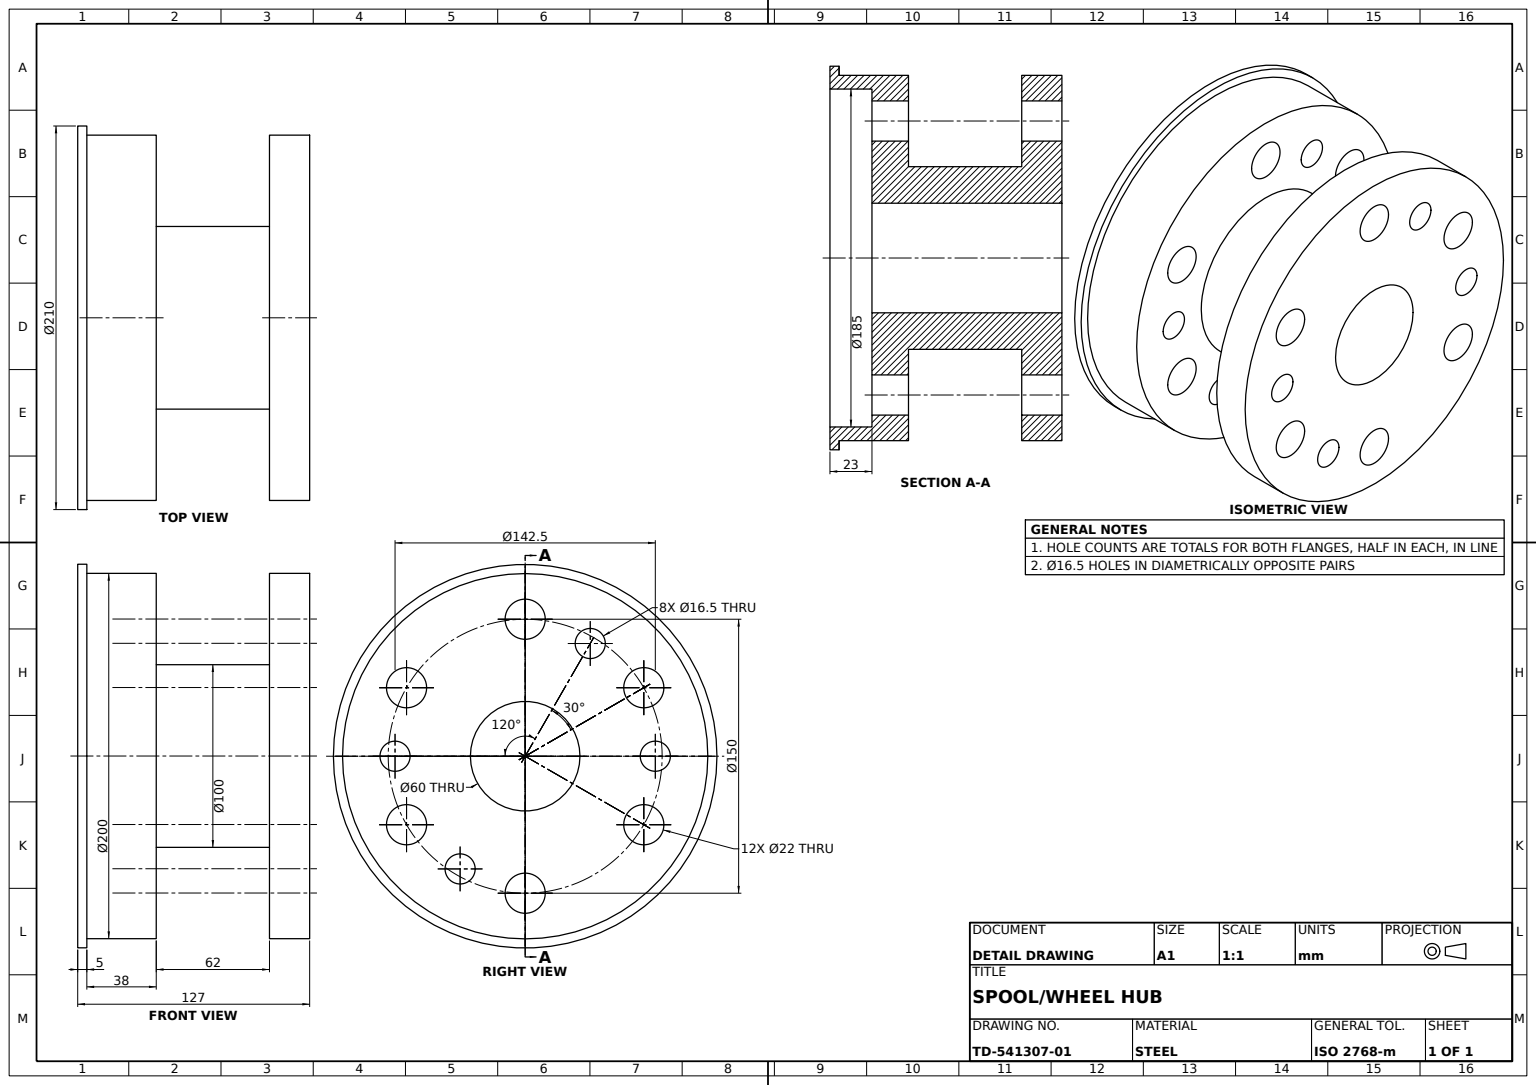
from build123d import *

# Parameters (mm, degrees)
RIM_LIP_SKETCH_210_R      = 105
RIM_LIP_210_DEPTH         = 5
FRONT_FLANGE_SKETCH_200_R = 100
FRONT_FLANGE_200_DEPTH    = 38
HUB_BARREL_SKETCH_100_R   = 50
HUB_BARREL_100_DEPTH      = 62
REAR_FLANGE_SKETCH_200_R  = 100
REAR_FLANGE_200_DEPTH     = 22
FRONT_RECESS_SKETCH_185_R = 92.5
FRONT_RECESS_185_DEPTH    = 23
BORE_SKETCH_60_R          = 30
BORE_60_DEPTH             = 182.289823211
FLANGE_HOLES_SKETCH_R     = 11
FLANGE_HOLES_SKETCH_R_2   = 8.25
FLANGE_HOLES_DEPTH        = 182.289823211


with BuildPart() as part:
    # Rim Lip Sketch Ø210 → Rim Lip Ø210 (new body)
    with BuildSketch(Plane.XY):
        Circle(RIM_LIP_SKETCH_210_R)
    extrude(amount=-RIM_LIP_210_DEPTH)

    # Front Flange Sketch Ø200 → Front Flange Ø200 (add)
    with BuildSketch(Plane(origin=(0, 0, -5), x_dir=(-1, 0, 0), z_dir=(0, 0, -1))):
        Circle(FRONT_FLANGE_SKETCH_200_R)
    extrude(amount=FRONT_FLANGE_200_DEPTH)

    # Hub Barrel Sketch Ø100 → Hub Barrel Ø100 (add)
    with BuildSketch(Plane(origin=(0, 0, -43), x_dir=(-1, 0, 0), z_dir=(0, 0, -1))):
        Circle(HUB_BARREL_SKETCH_100_R)
    extrude(amount=HUB_BARREL_100_DEPTH)

    # Rear Flange Sketch Ø200 → Rear Flange Ø200 (add)
    with BuildSketch(Plane(origin=(0, 0, -105), x_dir=(-1, 0, 0), z_dir=(0, 0, -1))):
        Circle(REAR_FLANGE_SKETCH_200_R)
    extrude(amount=REAR_FLANGE_200_DEPTH)

    # Front Recess Sketch Ø185 → Front Recess Ø185 (cut)
    with BuildSketch(Plane.XY):
        Circle(FRONT_RECESS_SKETCH_185_R)
    extrude(amount=-FRONT_RECESS_185_DEPTH, mode=Mode.SUBTRACT)

    # Bore Sketch Ø60 → Bore Ø60 (cut, through all)
    with BuildSketch(Plane.XY.offset(-23)):
        Circle(BORE_SKETCH_60_R)
    extrude(amount=-BORE_60_DEPTH, mode=Mode.SUBTRACT)

    # Flange Holes Sketch → Flange Holes (cut, through all)
    with BuildSketch(Plane.XY.offset(-23)):
        with Locations((0, 75)):
            Circle(FLANGE_HOLES_SKETCH_R)
        with Locations((64.951905284, 37.5)):
            Circle(FLANGE_HOLES_SKETCH_R)
        with Locations((64.951905284, -37.5)):
            Circle(FLANGE_HOLES_SKETCH_R)
        with Locations((0, -75)):
            Circle(FLANGE_HOLES_SKETCH_R)
        with Locations((-64.951905284, -37.5)):
            Circle(FLANGE_HOLES_SKETCH_R)
        with Locations((-64.951905284, 37.5)):
            Circle(FLANGE_HOLES_SKETCH_R)
        with Locations((-71.25, 0)):
            Circle(FLANGE_HOLES_SKETCH_R_2)
        with Locations((71.25, 0)):
            Circle(FLANGE_HOLES_SKETCH_R_2)
        with Locations((35.625, -61.70431002)):
            Circle(FLANGE_HOLES_SKETCH_R_2)
        with Locations((-35.625, 61.70431002)):
            Circle(FLANGE_HOLES_SKETCH_R_2)
    extrude(amount=-FLANGE_HOLES_DEPTH, mode=Mode.SUBTRACT)


solid = part.part
